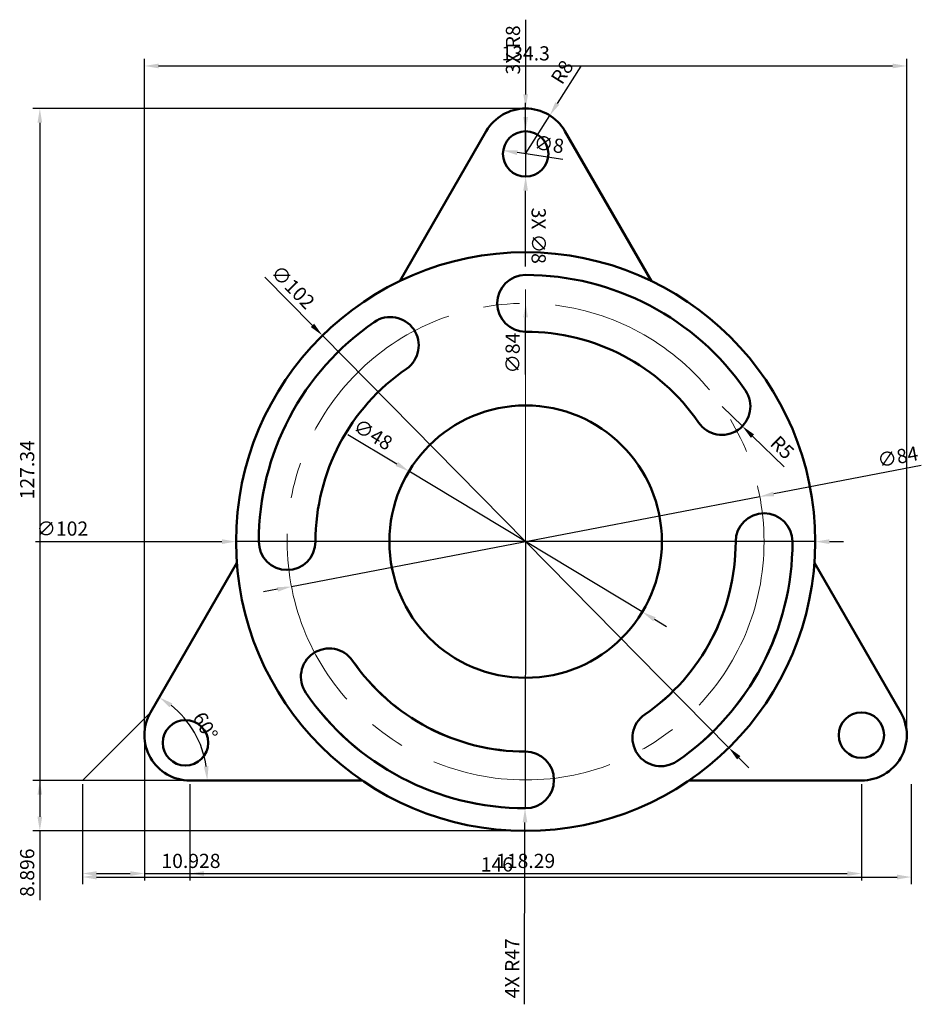
# Model space of a CAD drawing. Units: millimetres. Extents: x 92 to 251, y 91 to 265.
import ezdxf

# ---------------------------------------------------------------- set-up
doc = ezdxf.new("R2010")
doc.units = ezdxf.units.MM
doc.linetypes.add('CENTER', pattern=[50.8, 31.75, -6.35, 6.35, -6.35])
for name, color, linetype, lineweight in [('M-CNTR', 4, 'CENTER', 18), ('M-CONS', 8, 'Continuous', 13), ('M-DIMS', 2, 'Continuous', 25), ('M-OUTL', 7, 'Continuous', 50)]:
    doc.layers.add(name, color=color, linetype=linetype, lineweight=lineweight)
doc.styles.get("Standard").update_dxf_attribs({"font": 'arial.ttf'})
doc.dimstyles.new('ISO-25', dxfattribs={"dimtxt": 2.5, "dimasz": 2.5, "dimexe": 1.25, "dimexo": 0.625, "dimtad": 1, "dimtxsty": 'Standard', "dimcen": 2.5, "dimadec": 0, "dimazin": 0, "dimtfac": 1, "dimtmove": 0, "dimatfit": 3, "dimfxl": 1, "dimarcsym": 0})

# ---------------------------------------------------------------- blocks, each defined once
blk = doc.blocks.new('*U1')
for centre, radius, start, end in [((-17.29, 9.09), 5, 90, 270), ((-17.29, -32.91), 47, 34.5603, 90), ((-17.29, -32.91), 37, 34.5603, 90), ((17.29, -9.09), 5, 214.5603, 34.5603)]:
    blk.add_arc(centre, radius, start, end)
blk = doc.blocks.new('*U2')
at = {"layer": 'M-OUTL', "color": 0, "linetype": 'ByBlock', "lineweight": -2, "transparency": 16777216}
blk.add_blockref('*U1', (198.7, 205.63), dxfattribs=at)
for p, rotation in [((148.49, 190.01), 90.00000000000003), ((214.32, 155.42), 270), ((164.11, 139.8), 180)]:
    blk.add_blockref('*U1', p, dxfattribs=dict(at, rotation=rotation))
blk = doc.blocks.new('*D3')
at = {"layer": 'Defpoints', "color": 0, "transparency": 16777216}
for p in [(130.55, 168.96), (115.34, 142.61), (124.31, 136.4), (122.26, 130.61), (152.63, 130.61)]:
    blk.add_point(p, dxfattribs=at)
at = {"layer": 'M-DIMS', "color": 0, "lineweight": -2, "transparency": 16777216}
blk.add_arc((108.41, 130.61), 16.93, 8.4705, 51.5295, dxfattribs=at)
at = {"layer": 'M-DIMS', "color": 0, "transparency": 16777216}
for points in [[(118.7, 143.52), (119.17, 144.21), (116.87, 145.27)], [(125.56, 133.14), (124.73, 133.07), (125.33, 130.61)]]:
    blk.add_solid(points, dxfattribs=at)
at = {"layer": 'M-DIMS', "color": 0, "transparency": 16777216, "insert": (124.71, 140.03), "char_height": 2.5, "attachment_point": 5, "rotation": 300}
blk.add_mtext('60°', dxfattribs=at)
blk = doc.blocks.new('*D4')
at = {"layer": 'Defpoints', "color": 0, "transparency": 16777216}
for p in [(103.34, 130.61), (249.34, 130.61), (249.34, 113.6)]:
    blk.add_point(p, dxfattribs=at)
at = {"layer": 'M-DIMS', "color": 0, "lineweight": -2, "transparency": 16777216}
for p, q in [((103.34, 129.99), (103.34, 112.35)), ((249.34, 129.99), (249.34, 112.35)), ((105.84, 113.6), (246.84, 113.6))]:
    blk.add_line(p, q, dxfattribs=at)
at = {"layer": 'M-DIMS', "color": 0, "transparency": 16777216}
for points in [[(105.84, 114.02), (105.84, 113.18), (103.34, 113.6)], [(246.84, 114.02), (246.84, 113.18), (249.34, 113.6)]]:
    blk.add_solid(points, dxfattribs=at)
at = {"layer": 'M-DIMS', "color": 0, "transparency": 16777216, "insert": (176.34, 115.5), "char_height": 2.5, "attachment_point": 5}
blk.add_mtext('146', dxfattribs=at)
blk = doc.blocks.new('*D5')
at = {"layer": 'Defpoints', "color": 0, "transparency": 16777216}
for p in [(216, 196.54), (219.58, 193.06)]:
    blk.add_point(p, dxfattribs=at)
at = {"layer": 'M-DIMS', "color": 0, "lineweight": -2, "transparency": 16777216}
for p, q in [((216, 196.54), (219.58, 193.06)), ((226.96, 185.87), (221.37, 191.31))]:
    blk.add_line(p, q, dxfattribs=at)
at = {"layer": 'M-DIMS', "color": 0, "transparency": 16777216}
blk.add_solid([(221.66, 191.61), (221.08, 191.01), (219.58, 193.06)], dxfattribs=at)
at = {"layer": 'M-DIMS', "color": 0, "transparency": 16777216, "insert": (226.39, 189.08), "char_height": 2.5, "attachment_point": 5, "rotation": 315.8001}
blk.add_mtext('R5', dxfattribs=at)
blk = doc.blocks.new('*D6')
at = {"layer": 'Defpoints', "color": 0, "transparency": 16777216}
for p in [(145.61, 209.05), (217.2, 136.39)]:
    blk.add_point(p, dxfattribs=at)
at = {"layer": 'M-DIMS', "color": 0, "lineweight": -2, "transparency": 16777216}
for p, q in [((135.46, 219.35), (143.86, 210.83)), ((217.2, 136.39), (145.61, 209.05)), ((218.95, 134.6), (220.71, 132.82))]:
    blk.add_line(p, q, dxfattribs=at)
at = {"layer": 'M-DIMS', "color": 0, "transparency": 16777216}
for points in [[(144.16, 211.12), (143.56, 210.54), (145.61, 209.05)], [(219.25, 134.9), (218.66, 134.31), (217.2, 136.39)]]:
    blk.add_solid(points, dxfattribs=at)
at = {"layer": 'M-DIMS', "color": 0, "transparency": 16777216, "insert": (140.19, 217.36), "char_height": 2.5, "attachment_point": 5, "rotation": 314.5722}
blk.add_mtext('∅102', dxfattribs=at)
blk = doc.blocks.new('*D7')
at = {"layer": 'Defpoints', "color": 0, "transparency": 16777216}
for p in [(160.86, 185.11), (201.96, 160.32)]:
    blk.add_point(p, dxfattribs=at)
at = {"layer": 'M-DIMS', "color": 0, "lineweight": -2, "transparency": 16777216}
for p, q in [((150.1, 191.6), (158.71, 186.4)), ((201.96, 160.32), (160.86, 185.11)), ((204.1, 159.03), (206.24, 157.74))]:
    blk.add_line(p, q, dxfattribs=at)
at = {"layer": 'M-DIMS', "color": 0, "transparency": 16777216}
for points in [[(158.93, 186.76), (158.5, 186.05), (160.86, 185.11)], [(204.31, 159.39), (203.88, 158.67), (201.96, 160.32)]]:
    blk.add_solid(points, dxfattribs=at)
at = {"layer": 'M-DIMS', "color": 0, "transparency": 16777216, "insert": (154.36, 191.33), "char_height": 2.5, "attachment_point": 5, "rotation": 328.9048}
blk.add_mtext('∅48', dxfattribs=at)
blk = doc.blocks.new('*D8')
at = {"layer": 'Defpoints', "color": 0, "transparency": 16777216}
for p in [(181.41, 214.72), (181.41, 130.72)]:
    blk.add_point(p, dxfattribs=at)
at = {"layer": 'M-DIMS', "color": 0, "lineweight": -2, "transparency": 16777216}
blk.add_line((181.41, 202.18), (181.41, 212.22), dxfattribs=at)
at = {"layer": 'M-DIMS', "color": 0, "transparency": 16777216}
blk.add_solid([(180.99, 212.22), (181.82, 212.22), (181.41, 214.72)], dxfattribs=at)
at = {"layer": 'M-DIMS', "color": 0, "transparency": 16777216, "insert": (179.44, 205.95), "char_height": 2.5, "attachment_point": 5, "rotation": 90}
blk.add_mtext('∅84', dxfattribs=at)
blk = doc.blocks.new('*D9')
at = {"layer": 'Defpoints', "color": 0, "transparency": 16777216}
for p in [(177.45, 241.65), (185.36, 240.46)]:
    blk.add_point(p, dxfattribs=at)
at = {"layer": 'M-DIMS', "color": 0, "lineweight": -2, "transparency": 16777216}
blk.add_line((187.95, 240.07), (179.92, 241.28), dxfattribs=at)
at = {"layer": 'M-DIMS', "color": 0, "transparency": 16777216}
blk.add_solid([(179.99, 241.69), (179.86, 240.86), (177.45, 241.65)], dxfattribs=at)
at = {"layer": 'M-DIMS', "color": 0, "transparency": 16777216, "insert": (185.47, 242.43), "char_height": 2.5, "attachment_point": 5, "rotation": 351.4286}
blk.add_mtext('∅8', dxfattribs=at)
blk = doc.blocks.new('*D10')
at = {"layer": 'Defpoints', "color": 0, "transparency": 16777216}
for p in [(185.66, 247.83), (181.41, 241.05)]:
    blk.add_point(p, dxfattribs=at)
at = {"layer": 'M-DIMS', "color": 0, "lineweight": -2, "transparency": 16777216}
for p, q in [((191.12, 256.54), (186.99, 249.95)), ((181.41, 241.05), (185.66, 247.83))]:
    blk.add_line(p, q, dxfattribs=at)
at = {"layer": 'M-DIMS', "color": 0, "transparency": 16777216}
blk.add_solid([(186.63, 250.17), (187.34, 249.73), (185.66, 247.83)], dxfattribs=at)
at = {"layer": 'M-DIMS', "color": 0, "transparency": 16777216, "insert": (188.11, 255.31), "char_height": 2.5, "attachment_point": 5, "rotation": 57.9074}
blk.add_mtext('R8', dxfattribs=at)
blk = doc.blocks.new('MOUNT-HOLE-D8')
blk.add_circle((4, 4), 4)
blk = doc.blocks.new('*D12')
at = {"layer": 'Defpoints', "color": 0, "transparency": 16777216}
for p in [(248.55, 256.55), (114.26, 138.61), (248.55, 138.61)]:
    blk.add_point(p, dxfattribs=at)
at = {"layer": 'M-DIMS', "color": 0, "lineweight": -2, "transparency": 16777216}
for p, q in [((114.26, 139.24), (114.26, 257.8)), ((248.55, 139.24), (248.55, 257.8)), ((116.76, 256.55), (246.05, 256.55))]:
    blk.add_line(p, q, dxfattribs=at)
at = {"layer": 'M-DIMS', "color": 0, "transparency": 16777216}
for points in [[(116.76, 256.97), (116.76, 256.14), (114.26, 256.55)], [(246.05, 256.97), (246.05, 256.14), (248.55, 256.55)]]:
    blk.add_solid(points, dxfattribs=at)
at = {"layer": 'M-DIMS', "color": 0, "transparency": 16777216, "insert": (181.41, 258.45), "char_height": 2.5, "attachment_point": 5}
blk.add_mtext('134.3', dxfattribs=at)
blk = doc.blocks.new('*D13')
at = {"layer": 'Defpoints', "color": 0, "transparency": 16777216}
for p in [(181.41, 249.05), (95.84, 121.72), (181.41, 121.72)]:
    blk.add_point(p, dxfattribs=at)
at = {"layer": 'M-DIMS', "color": 0, "lineweight": -2, "transparency": 16777216}
for p, q in [((180.78, 249.05), (94.59, 249.05)), ((95.84, 246.55), (95.84, 124.22)), ((180.78, 121.72), (94.59, 121.72))]:
    blk.add_line(p, q, dxfattribs=at)
at = {"layer": 'M-DIMS', "color": 0, "transparency": 16777216}
for points in [[(95.42, 246.55), (96.25, 246.55), (95.84, 249.05)], [(95.42, 124.22), (96.25, 124.22), (95.84, 121.72)]]:
    blk.add_solid(points, dxfattribs=at)
at = {"layer": 'M-DIMS', "color": 0, "transparency": 16777216, "insert": (93.93, 185.38), "char_height": 2.5, "attachment_point": 5, "rotation": 90}
blk.add_mtext('127.34', dxfattribs=at)
blk = doc.blocks.new('*D14')
at = {"layer": 'Defpoints', "color": 0, "transparency": 16777216}
for p in [(152.63, 130.61), (95.84, 121.72), (181.41, 121.72)]:
    blk.add_point(p, dxfattribs=at)
at = {"layer": 'M-DIMS', "color": 0, "lineweight": -2, "transparency": 16777216}
for p, q in [((152, 130.61), (94.59, 130.61)), ((95.84, 128.11), (95.84, 124.22)), ((180.78, 121.72), (94.59, 121.72)), ((95.84, 121.72), (95.84, 109.53))]:
    blk.add_line(p, q, dxfattribs=at)
at = {"layer": 'M-DIMS', "color": 0, "transparency": 16777216}
for points in [[(95.42, 128.11), (96.25, 128.11), (95.84, 130.61)], [(95.42, 124.22), (96.25, 124.22), (95.84, 121.72)]]:
    blk.add_solid(points, dxfattribs=at)
at = {"layer": 'M-DIMS', "color": 0, "transparency": 16777216, "insert": (93.93, 114.37), "char_height": 2.5, "attachment_point": 5, "rotation": 90}
blk.add_mtext('8.896', dxfattribs=at)
blk = doc.blocks.new('*D15')
at = {"layer": 'Defpoints', "color": 0, "transparency": 16777216}
for p in [(122.26, 130.61), (240.55, 130.61), (240.55, 114.22)]:
    blk.add_point(p, dxfattribs=at)
at = {"layer": 'M-DIMS', "color": 0, "lineweight": -2, "transparency": 16777216}
for p, q in [((122.26, 129.99), (122.26, 112.97)), ((240.55, 129.99), (240.55, 112.97)), ((124.76, 114.22), (238.05, 114.22))]:
    blk.add_line(p, q, dxfattribs=at)
at = {"layer": 'M-DIMS', "color": 0, "transparency": 16777216}
for points in [[(124.76, 114.63), (124.76, 113.8), (122.26, 114.22)], [(238.05, 114.63), (238.05, 113.8), (240.55, 114.22)]]:
    blk.add_solid(points, dxfattribs=at)
at = {"layer": 'M-DIMS', "color": 0, "transparency": 16777216, "insert": (181.41, 116.12), "char_height": 2.5, "attachment_point": 5}
blk.add_mtext('118.29', dxfattribs=at)
blk = doc.blocks.new('*D16')
at = {"layer": 'Defpoints', "color": 0, "transparency": 16777216}
for p in [(114.26, 138.61), (103.34, 130.61), (114.26, 114.22)]:
    blk.add_point(p, dxfattribs=at)
at = {"layer": 'M-DIMS', "color": 0, "lineweight": -2, "transparency": 16777216}
for p, q in [((114.26, 137.99), (114.26, 112.97)), ((103.34, 129.99), (103.34, 112.97)), ((105.84, 114.22), (111.76, 114.22)), ((114.26, 114.22), (128.16, 114.22))]:
    blk.add_line(p, q, dxfattribs=at)
at = {"layer": 'M-DIMS', "color": 0, "transparency": 16777216}
for points in [[(105.84, 114.63), (105.84, 113.8), (103.34, 114.22)], [(111.76, 114.63), (111.76, 113.8), (114.26, 114.22)]]:
    blk.add_solid(points, dxfattribs=at)
at = {"layer": 'M-DIMS', "color": 0, "transparency": 16777216, "insert": (122.46, 116.12), "char_height": 2.5, "attachment_point": 5}
blk.add_mtext('10.928', dxfattribs=at)
blk = doc.blocks.new('*D17')
at = {"layer": 'Defpoints', "color": 0, "transparency": 16777216}
for p in [(130.41, 172.72), (232.41, 172.72)]:
    blk.add_point(p, dxfattribs=at)
at = {"layer": 'M-DIMS', "color": 0, "lineweight": -2, "transparency": 16777216}
for p, q in [((95.07, 172.72), (127.91, 172.72)), ((232.41, 172.72), (130.41, 172.72)), ((234.91, 172.72), (237.41, 172.72))]:
    blk.add_line(p, q, dxfattribs=at)
at = {"layer": 'M-DIMS', "color": 0, "transparency": 16777216}
for points in [[(127.91, 173.13), (127.91, 172.3), (130.41, 172.72)], [(234.91, 173.13), (234.91, 172.3), (232.41, 172.72)]]:
    blk.add_solid(points, dxfattribs=at)
at = {"layer": 'M-DIMS', "color": 0, "transparency": 16777216, "insert": (99.81, 174.69), "char_height": 2.5, "attachment_point": 5, "rotation": 0.0001}
blk.add_mtext('∅102', dxfattribs=at)
blk = doc.blocks.new('*D18')
at = {"layer": 'Defpoints', "color": 0, "transparency": 16777216}
for p in [(222.65, 180.65), (140.16, 164.78)]:
    blk.add_point(p, dxfattribs=at)
at = {"layer": 'M-DIMS', "color": 0, "lineweight": -2, "transparency": 16777216}
for p, q in [((251.1, 186.12), (225.11, 181.12)), ((140.16, 164.78), (222.65, 180.65)), ((137.71, 164.31), (135.25, 163.84))]:
    blk.add_line(p, q, dxfattribs=at)
at = {"layer": 'M-DIMS', "color": 0, "transparency": 16777216}
for points in [[(225.03, 181.53), (225.18, 180.71), (222.65, 180.65)], [(137.63, 164.72), (137.79, 163.9), (140.16, 164.78)]]:
    blk.add_solid(points, dxfattribs=at)
at = {"layer": 'M-DIMS', "color": 0, "transparency": 16777216, "insert": (247.02, 187.35), "char_height": 2.5, "attachment_point": 5, "rotation": 10.8889}
blk.add_mtext('∅84', dxfattribs=at)
blk = doc.blocks.new('*D19')
at = {"layer": 'Defpoints', "color": 0, "transparency": 16777216}
for p in [(181.41, 245.05), (181.41, 237.05)]:
    blk.add_point(p, dxfattribs=at)
at = {"layer": 'M-DIMS', "color": 0, "lineweight": -2, "transparency": 16777216}
for p, q in [((181.41, 247.55), (181.41, 250.05)), ((181.41, 245.05), (181.41, 237.05)), ((181.41, 221.2), (181.41, 234.55))]:
    blk.add_line(p, q, dxfattribs=at)
at = {"layer": 'M-DIMS', "color": 0, "transparency": 16777216}
for points in [[(181.82, 247.55), (180.99, 247.55), (181.41, 245.05)], [(181.82, 234.55), (180.99, 234.55), (181.41, 237.05)]]:
    blk.add_solid(points, dxfattribs=at)
at = {"layer": 'M-DIMS', "color": 0, "transparency": 16777216, "insert": (183.38, 226.63), "char_height": 2.5, "attachment_point": 5, "rotation": 270.0023}
blk.add_mtext('3X ∅8', dxfattribs=at)
blk = doc.blocks.new('*D20')
at = {"layer": 'Defpoints', "color": 0, "transparency": 16777216}
for p in [(181.41, 249.05), (181.41, 241.05)]:
    blk.add_point(p, dxfattribs=at)
at = {"layer": 'M-DIMS', "color": 0, "lineweight": -2, "transparency": 16777216}
for p, q in [((181.41, 264.71), (181.41, 251.55)), ((181.41, 241.05), (181.41, 249.05))]:
    blk.add_line(p, q, dxfattribs=at)
at = {"layer": 'M-DIMS', "color": 0, "transparency": 16777216}
blk.add_solid([(180.99, 251.55), (181.82, 251.55), (181.41, 249.05)], dxfattribs=at)
at = {"layer": 'M-DIMS', "color": 0, "transparency": 16777216, "insert": (179.5, 259.38), "char_height": 2.5, "attachment_point": 5, "rotation": 90}
blk.add_mtext('3X R8', dxfattribs=at)
blk = doc.blocks.new('*D21')
at = {"layer": 'Defpoints', "color": 0, "transparency": 16777216}
for p in [(181.41, 172.72), (181.3, 125.72)]:
    blk.add_point(p, dxfattribs=at)
at = {"layer": 'M-DIMS', "color": 0, "lineweight": -2, "transparency": 16777216}
for p, q in [((181.41, 172.72), (181.3, 125.72)), ((181.22, 91.17), (181.29, 123.22))]:
    blk.add_line(p, q, dxfattribs=at)
at = {"layer": 'M-DIMS', "color": 0, "transparency": 16777216}
blk.add_solid([(180.88, 123.22), (181.71, 123.22), (181.3, 125.72)], dxfattribs=at)
at = {"layer": 'M-DIMS', "color": 0, "transparency": 16777216, "insert": (179.36, 97.52), "char_height": 2.5, "attachment_point": 5, "rotation": 89.8698}
blk.add_mtext('4X R47', dxfattribs=at)

msp = doc.modelspace()

# ---------------------------------------------------------------- linework, layer by layer
at = {"layer": 'M-CNTR'}
for q in [(181.4068, 223.7161), (130.4068, 172.7161), (181.4068, 121.7161), (232.4068, 172.7161)]:
    msp.add_line((181.4068, 172.7161), q, dxfattribs=at)
msp.add_circle((181.4068, 172.7161), 42, dxfattribs=at)
at = {"layer": 'M-CONS'}
for p in [(115.335, 142.6122), (122.2632, 130.6122)]:
    msp.add_line(p, (103.335, 130.6122), dxfattribs=at)
at = {"layer": 'M-OUTL'}
for p, q in [((174.4786, 245.0519), (159.2312, 218.6425)), ((203.5825, 218.6425), (188.335, 245.0519)), ((130.5455, 168.9575), (115.335, 142.6122)), ((247.4786, 142.6122), (232.2682, 168.9575)), ((122.2632, 130.6122), (152.6273, 130.6122)), ((210.1864, 130.6122), (240.5504, 130.6122))]:
    msp.add_line(p, q, dxfattribs=at)
for radius in [51, 24]:
    msp.add_circle((181.4068, 172.7161), radius, dxfattribs=at)
for centre, radius, start, end in [((181.4068, 241.0519), 8, 30, 150), ((181.4068, 172.7161), 37, 304.560322, 0), ((181.4068, 172.7161), 47, 304.560322, 0), ((181.4068, 172.7161), 37, 214.560322, 270), ((181.4068, 172.7161), 47, 214.560322, 270), ((122.2632, 138.6122), 8, 150, 270), ((240.5504, 138.6122), 8, 270, 30)]:
    msp.add_arc(centre, radius, start, end, dxfattribs=at)

# ---------------------------------------------------------------- block references
for name, p in [('MOUNT-HOLE-D8', (177.407, 237.052)), ('*U2', (0, 0)), ('MOUNT-HOLE-D8', (236.5506, 134.6123)), ('MOUNT-HOLE-D8', (117.4815, 133.258))]:
    msp.add_blockref(name, p, dxfattribs=at)

# ---------------------------------------------------------------- dimensions: what is measured, and where the dimension line sits
at = {"layer": 'M-DIMS'}
dim = msp.add_radius_dim(center=(181.4068, 241.0519), mpoint=(181.4068, 249.0519), text='3X <>', dimstyle='ISO-25', override={"dimdec": 0, "dimlfac": 1, "dimrnd": 0, "dimzin": 0, "dimdsep": 46, "dimlunit": 2}, dxfattribs=at)
dim.commit()
dim.dimension.update_dxf_attribs({"geometry": '*D20', "text_midpoint": (179.5046, 259.3802)})
for base, p1, p2, override, picture, middle in [((248.5504, 256.5519), (114.2632, 138.6122), (248.5504, 138.6122), {"dimdec": 1, "dimlfac": 1, "dimrnd": 0, "dimzin": 0, "dimdsep": 46, "dimlunit": 2}, '*D12', (181.4068, 258.4542)), ((114.2632, 114.2161), (103.335, 130.6122), (114.2632, 138.6122), {"dimdec": 3, "dimlfac": 1, "dimrnd": 0, "dimzin": 0, "dimdsep": 46, "dimlunit": 2}, '*D16', (122.4624, 116.1175)), ((249.335, 113.6002), (103.335, 130.6122), (249.335, 130.6122), {"dimclrd": 0, "dimclre": 0, "dimclrt": 0}, '*D4', (176.335, 115.5017)), ((240.5504, 114.2161), (122.2632, 130.6122), (240.5504, 130.6122), {"dimdec": 2, "dimlfac": 1, "dimrnd": 0, "dimzin": 0, "dimdsep": 46, "dimlunit": 2}, '*D15', (181.4068, 116.1175))]:
    dim = msp.add_linear_dim(base=base, p1=p1, p2=p2, dimstyle='ISO-25', override=override, dxfattribs=at)
    dim.commit()
    dim.dimension.update_dxf_attribs({"geometry": picture, "text_midpoint": middle})
for center, mpoint, picture, middle in [((181.4068, 241.0519), (185.6572, 247.8294), '*D10', (188.1071, 255.3149)), ((215.9951, 196.5416), (219.5796, 193.0557), '*D5', (226.3861, 189.0819))]:
    dim = msp.add_radius_dim(center=center, mpoint=mpoint, dimstyle='ISO-25', override={"dimclrd": 0, "dimclre": 0, "dimclrt": 0}, dxfattribs=at)
    dim.commit()
    dim.dimension.update_dxf_attribs({"geometry": picture, "text_midpoint": middle})
dim = msp.add_diameter_dim_2p(p1=(181.4067, 245.0519), p2=(181.407, 237.0519), text='3X <>', dimstyle='ISO-25', override={"dimdec": 0, "dimlfac": 1, "dimrnd": 0, "dimzin": 0, "dimdsep": 46, "dimlunit": 2}, dxfattribs=at)
dim.commit()
dim.dimension.update_dxf_attribs({"geometry": '*D19', "text_midpoint": (181.4074, 226.6264), "dimtype": 163})
for p1, override, picture, middle in [((181.4068, 249.0519), {"dimdec": 2, "dimlfac": 1, "dimrnd": 0, "dimzin": 0, "dimdsep": 46, "dimlunit": 2}, '*D13', (93.9328, 185.384)), ((152.6273, 130.6122), {"dimdec": 3, "dimlfac": 1, "dimrnd": 0, "dimzin": 0, "dimdsep": 46, "dimlunit": 2}, '*D14', (93.9336, 114.3721))]:
    dim = msp.add_linear_dim(base=(95.835, 121.7161), p1=p1, p2=(181.4068, 121.7161), angle=90, dimstyle='ISO-25', override=override, dxfattribs=at)
    dim.commit()
    dim.dimension.update_dxf_attribs({"geometry": picture, "text_midpoint": middle})
for p1, p2, override, picture, middle in [((185.3622, 240.4557), (177.4515, 241.6481), {"dimclrd": 0, "dimclre": 0, "dimclrt": 0}, '*D9', (185.1713, 240.4845)), ((181.4068, 130.7161), (181.4068, 214.7161), {"dimclrd": 0, "dimclre": 0, "dimclrt": 0}, '*D8', (181.4068, 205.9456)), ((201.9583, 160.321), (160.8554, 185.1111), {"dimclrd": 0, "dimclre": 0, "dimclrt": 0}, '*D7', (153.3386, 189.6447)), ((140.163, 164.782), (222.6506, 180.6501), {"dimdec": 0, "dimlfac": 1, "dimrnd": 0, "dimzin": 0, "dimdsep": 46, "dimlunit": 2}, '*D18', (247.3969, 185.4106)), ((232.4068, 172.7161), (130.4068, 172.716), {"dimdec": 0, "dimlfac": 1, "dimrnd": 0, "dimzin": 0, "dimdsep": 46, "dimlunit": 2}, '*D17', (99.8068, 172.716))]:
    dim = msp.add_diameter_dim_2p(p1=p1, p2=p2, dimstyle='ISO-25', override=override, dxfattribs=at)
    dim.commit()
    dim.dimension.update_dxf_attribs({"geometry": picture, "text_midpoint": middle, "dimtype": 163})
dim = msp.add_diameter_dim_2p(p1=(217.199, 136.3854), p2=(145.6147, 209.0468), dimstyle='ISO-25', override={"dimclrd": 0, "dimclre": 0, "dimclrt": 0}, dxfattribs=at)
dim.commit()
dim.dimension.update_dxf_attribs({"geometry": '*D6', "text_midpoint": (140.1876, 217.3645)})
dim = msp.add_radius_dim(center=(181.4068, 172.7161), mpoint=(181.3, 125.7162), text='4X <>', dimstyle='ISO-25', override={"dimdec": 0, "dimlfac": 1, "dimrnd": 0, "dimzin": 0, "dimdsep": 46, "dimlunit": 2}, dxfattribs=at)
dim.commit()
dim.dimension.update_dxf_attribs({"geometry": '*D21', "text_midpoint": (181.2359, 97.5163), "dimtype": 164})
dim = msp.add_angular_dim_2l(base=(124.3118, 136.4011), line1=((122.2632, 130.6122), (152.6273, 130.6122)), line2=((130.5455, 168.9575), (115.335, 142.6122)), dimstyle='ISO-25', override={"dimclrd": 0, "dimclre": 0, "dimclrt": 0}, dxfattribs=at)
dim.commit()
dim.dimension.update_dxf_attribs({"geometry": '*D3', "text_midpoint": (124.7116, 140.0258)})

doc.saveas('drawing.dxf')
